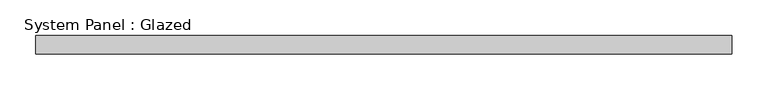
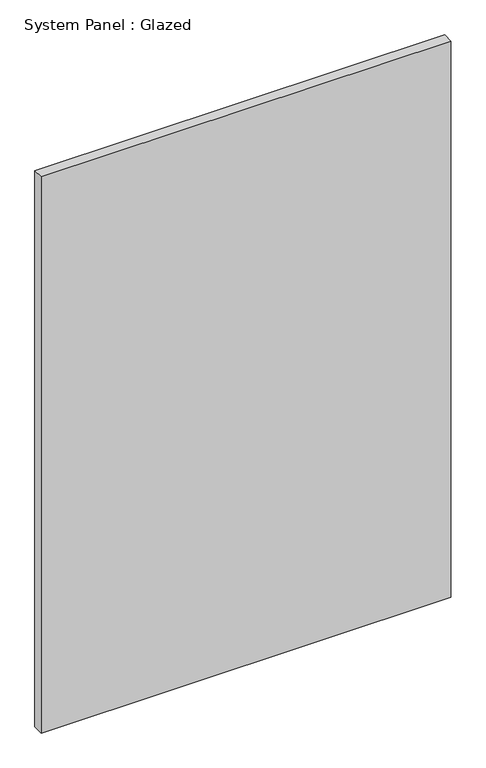
"""IFC4 building model written with IfcOpenShell, lengths in millimetres: plate geometry, System Panel : Glazed."""

from ifc_helpers import new_model, si_unit, origin, origin_with_axes, place, context, project, spatial, polyline, outline, extrude, source, transform, mapped, element, save


def system_panel_glazed_63a83b1f(model_context):
    return source(origin(), model_context, "Body", "SweptSolid", [
        extrude(outline(polyline([(485.775, 19.05), (-485.775, 19.05), (-485.775, 44.45), (485.775, 44.45), (485.775, 19.05)])), origin_with_axes(), (0.0, 0.0, 1.0), 1394.1896321),
    ])


if __name__ == "__main__":
    model = new_model("IFC4")
    model_context = context("Model", 3, world=origin())
    ifc_project = project(units=[si_unit("LENGTHUNIT", "METRE", prefix="MILLI")], contexts=[model_context])
    site = spatial("IfcSite", under=ifc_project)
    building = spatial("IfcBuilding", under=site)
    placement = place(None, origin())
    system_panel_glazed_shape = system_panel_glazed_63a83b1f(model_context)
    element("IfcPlate", 1, ObjectType="System Panel : Glazed", at=placement, inside=building, context=model_context, shape_type="MappedRepresentation", body=[
        mapped(system_panel_glazed_shape, transform((0.0, 0.0, 0.0), x_axis=(1.0, 0.0, 0.0), y_axis=(0.0, 1.0, 0.0), z_axis=(0.0, 0.0, 1.0))),
    ])
    save(model, "model.ifc")

# Revit data of these elements
# Type "System Panel : Glazed"
#   Construction Type Id = "GSP4R"
#   Analytic Construction = "1/8 in Pilkington single glazing"
#   Visual Light Transmittance = 0.9
#   Solar Heat Gain Coefficient = 0.86
#   Heat Transfer Coefficient (U) = 1.18115 BTU/(h·ft²·°F)
#   Define Thermal Properties by = 1
# Element 1 (IfcPlate, "System Panel : Glazed")
#   Materials on its faces: "Glass"
# Materials
#   "Glass": class "Glass", colour RGB 0 128 192, transparency 0.75, Description = "Soda Lime Glass", Cost = 0
